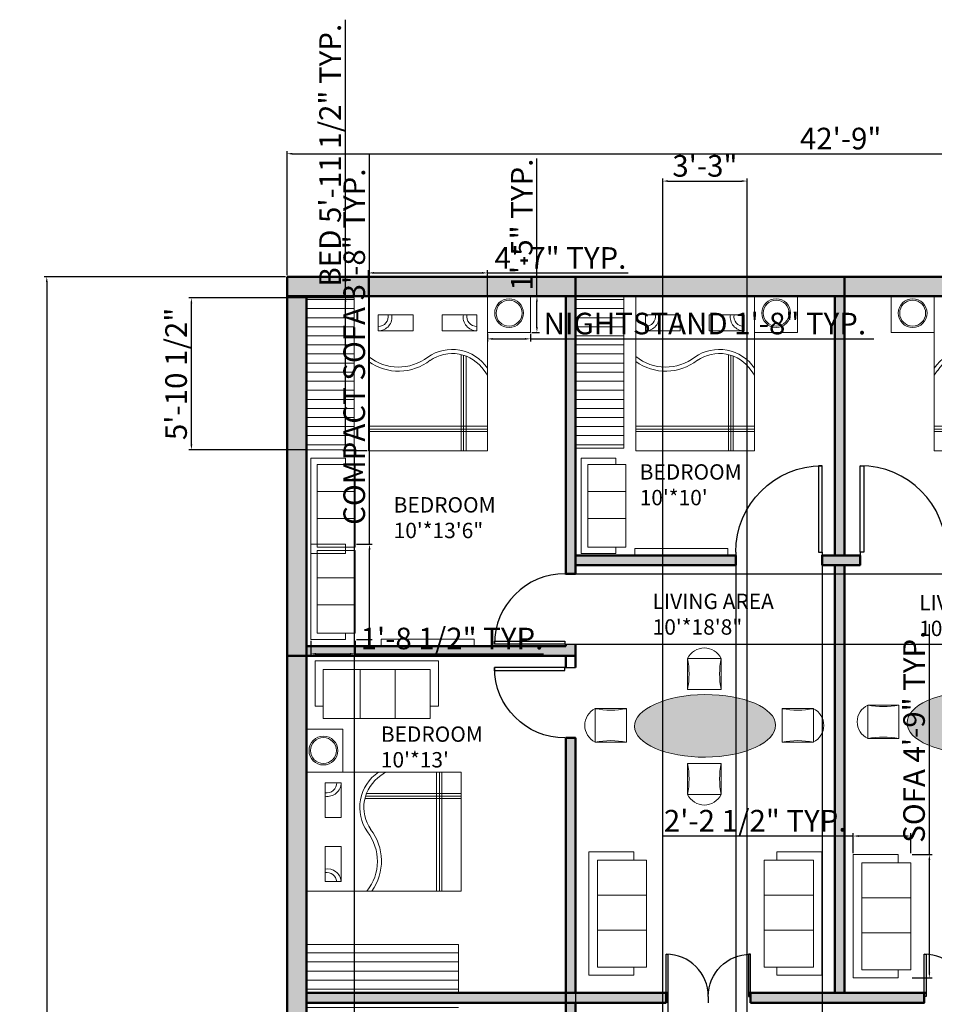
# Model space of a CAD drawing. Units: inches. Extents: x 1477 to 2233, y 1388 to 2326.
# Tile 3 of 4: x 1477 to 1901, y 1870 to 2326. Entities that reach past the tile are written whole.
import ezdxf

# ---------------------------------------------------------------- set-up
doc = ezdxf.new("R2010")
doc.units = ezdxf.units.IN
for name, color, linetype, lineweight in [('A-ANNO-DIMS', 2, 'Continuous', 18), ('A-AREA-IDEN', 7, 'Continuous', 18), ('A-DOOR', 4, 'Continuous', 25), ('A-EQPM', 8, 'Continuous', 18), ('A-FURN-PATT', 9, 'Continuous', 13), ('A-WALL-PATT', 10, 'Continuous', 13), ('bed', 200, 'Continuous', 18), ('book', 104, 'Continuous', 18), ('dining', 220, 'Continuous', 18), ('sofa', 130, 'Continuous', 18), ('table', 40, 'Continuous', 18), ('wall', 10, 'Continuous', 50)]:
    doc.layers.add(name, color=color, linetype=linetype, lineweight=lineweight)
doc.styles.get("Standard").update_dxf_attribs({"font": 'arial.ttf'})
doc.dimstyles.new('ISO-25', dxfattribs={"dimtxt": 10, "dimasz": 2.5, "dimexe": 1.25, "dimexo": 0.625, "dimtad": 1, "dimdec": 0, "dimlunit": 4, "dimtxsty": 'Standard', "dimcen": 2.5, "dimadec": 0, "dimazin": 0, "dimtfac": 1, "dimtdec": 0, "dimtmove": 0, "dimatfit": 3, "dimfxl": 1, "dimarcsym": 0})

# ---------------------------------------------------------------- blocks, each defined once
blk = doc.blocks.new('*U2')
for p, q in [((0, 0), (0, -6)), ((40, 0), (40, -6))]:
    blk.add_line(p, q)
blk.add_lwpolyline([(0, 0), (0, 40), (1.75, 40), (1.75, 0)], close=True)
blk.add_arc((0, 0), 40, 0, 90)
blk = doc.blocks.new('*D4')
at = {"layer": 'A-ANNO-DIMS', "color": 0, "lineweight": -2, "transparency": 16777216}
for p, q in [((1601.11, 2207.8), (1601.11, 2265.33)), ((2113.61, 2207.8), (2113.61, 2265.33)), ((1603.61, 2264.08), (2111.11, 2264.08))]:
    blk.add_line(p, q, dxfattribs=at)
at = {"layer": 'A-ANNO-DIMS', "color": 0, "transparency": 16777216}
for points in [[(1603.61, 2264.5), (1603.61, 2263.66), (1601.11, 2264.08)], [(2111.11, 2264.5), (2111.11, 2263.66), (2113.61, 2264.08)]]:
    blk.add_solid(points, dxfattribs=at)
at = {"layer": 'Defpoints', "color": 0, "transparency": 16777216}
for p in [(2113.61, 2264.08), (1601.11, 2207.17), (2113.61, 2207.17)]:
    blk.add_point(p, dxfattribs=at)
at = {"layer": 'A-ANNO-DIMS', "color": 0, "transparency": 16777216, "insert": (1857.36, 2269.81), "char_height": 10, "attachment_point": 5}
blk.add_mtext('42\'-9"', dxfattribs=at)
blk = doc.blocks.new('*D5')
at = {"layer": 'A-ANNO-DIMS', "color": 0, "lineweight": -2, "transparency": 16777216}
for p, q in [((1600.48, 2207.17), (1488.68, 2207.17)), ((1489.93, 2204.67), (1489.93, 1443.67)), ((1600.48, 1441.17), (1488.68, 1441.17))]:
    blk.add_line(p, q, dxfattribs=at)
at = {"layer": 'A-ANNO-DIMS', "color": 0, "transparency": 16777216}
for points in [[(1489.51, 2204.67), (1490.35, 2204.67), (1489.93, 2207.17)], [(1489.51, 1443.67), (1490.35, 1443.67), (1489.93, 1441.17)]]:
    blk.add_solid(points, dxfattribs=at)
at = {"layer": 'Defpoints', "color": 0, "transparency": 16777216}
for p in [(1601.11, 2207.17), (1489.93, 1441.17), (1601.11, 1441.17)]:
    blk.add_point(p, dxfattribs=at)
at = {"layer": 'A-ANNO-DIMS', "color": 0, "transparency": 16777216, "insert": (1484.2, 1824.17), "char_height": 10, "attachment_point": 5, "rotation": 90}
blk.add_mtext('63\'-10"', dxfattribs=at)
blk = doc.blocks.new('BED-DOUBLE')
for p, q in [((42.9, 44.24), (42.9, 44.54)), ((42.9, 44.24), (42.9, 0)), ((43.98, 44.24), (43.98, 0)), ((45.09, 43.85), (45.09, 0)), ((53.44, 37.23), (54.99, 35.03)), ((0, 11.42), (54.99, 11.42)), ((0, 10.1), (54.99, 10.1)), ((0, 8.97), (54.99, 8.97))]:
    blk.add_line(p, q)
for points in [[(0, 71.61), (54.99, 71.61), (54.99, 0), (0, 0)], [(4.46, 63.01), (20.6, 63.01), (20.6, 55.57), (4.46, 55.57)], [(50.13, 63.01), (34, 63.01), (34, 55.57), (50.13, 55.57)]]:
    blk.add_lwpolyline(points, close=True)
for centre, radius, start, end in [((4.46, 61.93), 6.36, 270, 9.8305), ((4.46, 62.26), 4.68, 270, 9.2541), ((50.13, 61.93), 6.36, 170.1695, 270), ((50.13, 62.26), 4.68, 170.7459, 270), ((38.65, 27.17), 19.76, 34.2245, 124.798), ((13.85, 60.88), 22.1, 231.1871, 307.7214), ((13.85, 60.88), 23.99, 234.7235, 307.7214), ((38.65, 27.17), 17.88, 34.2245, 124.798)]:
    blk.add_arc(centre, radius, start, end)
blk = doc.blocks.new('BED-DOUBLE-ALT')
for p, q in [((8.97, 0), (8.97, 54.99)), ((10.1, 0), (10.1, 54.99)), ((11.42, 0), (11.42, 54.99)), ((37.23, 53.44), (35.03, 54.99)), ((43.85, 45.09), (0, 45.09)), ((44.24, 43.98), (0, 43.98)), ((44.24, 42.9), (0, 42.9)), ((44.24, 42.9), (44.54, 42.9))]:
    blk.add_line(p, q)
for points in [[(71.61, 0), (71.61, 54.99), (0, 54.99), (0, 0)], [(63.01, 50.13), (63.01, 34), (55.57, 34), (55.57, 50.13)], [(63.01, 4.46), (63.01, 20.6), (55.57, 20.6), (55.57, 4.46)]]:
    blk.add_lwpolyline(points, close=True)
for centre, radius, start, end in [((27.17, 38.65), 19.76, 325.202, 55.7755), ((27.17, 38.65), 17.88, 325.202, 55.7755), ((61.93, 50.13), 6.36, 180, 279.8305), ((62.26, 50.13), 4.68, 180, 279.2541), ((60.88, 13.85), 23.99, 142.2786, 215.2765), ((60.88, 13.85), 22.1, 142.2786, 218.8129), ((61.93, 3.93), 6.36, 80.1695, 175.1865), ((62.26, 3.93), 4.68, 80.7459, 173.4549)]:
    blk.add_arc(centre, radius, start, end)
blk = doc.blocks.new('NIGHTSTAND-LAMP')
blk.add_lwpolyline([(0, 16.8), (19.92, 16.8), (19.92, 0), (0, 0)], close=True)
for radius in [6.66, 6]:
    blk.add_circle((10.02, 8.94), radius)
blk = doc.blocks.new('SOFA-COMPACT')
for p, q in [((0, 0), (0, 44.13)), ((16.12, 44.13), (0, 44.13)), ((16.12, 41.13), (16.12, 44.13)), ((3.06, 28.6), (20.62, 28.6)), ((3.06, 16.11), (20.62, 16.11)), ((16.12, 2.91), (16.12, 0)), ((16.12, 0), (0, 0))]:
    blk.add_line(p, q)
blk.add_lwpolyline([(20.62, 2.91), (3.06, 2.91), (3.06, 41.13), (20.62, 41.13)], close=True)
blk = doc.blocks.new('SOFA-COMPACT-ALT')
for p, q in [((0, 4.5), (0, 20.62)), ((0, 20.62), (44.13, 20.62)), ((44.13, 4.5), (44.13, 20.62)), ((16.11, 17.56), (16.11, 0)), ((28.61, 17.56), (28.61, 0)), ((2.91, 4.5), (0, 4.5)), ((1.29, 4.5), (2.91, 4.5)), ((41.13, 4.5), (44.13, 4.5))]:
    blk.add_line(p, q)
blk.add_lwpolyline([(2.91, 0), (2.91, 17.56), (41.13, 17.56), (41.13, 0)], close=True)
blk = doc.blocks.new('SOFA-STANDARD-ALT')
for p, q in [((0, 26.7), (57.14, 26.7)), ((0, 26.7), (0, 5.83)), ((57.14, 5.83), (57.14, 26.7)), ((20.86, 22.74), (20.86, 0)), ((37.04, 22.74), (37.04, 0)), ((3.76, 5.83), (0, 5.83)), ((53.26, 5.83), (57.14, 5.83))]:
    blk.add_line(p, q)
blk.add_lwpolyline([(3.76, 0), (3.76, 22.74), (53.26, 22.74), (53.26, 0)], close=True)
blk = doc.blocks.new('CHAIR-DINING')
blk.add_lwpolyline([(0, 0), (15.48, 0), (15.48, 14.4), (0, 14.4)], close=True)
for centre, radius, start, end in [((7.74, 10.64), 8.6, 25.8733, 154.1267), ((-38.59, 7.2), 39.26, 349.434, 10.566), ((53.9, 7.2), 39.09, 169.3873, 190.6127)]:
    blk.add_arc(centre, radius, start, end)
blk = doc.blocks.new('*D17')
at = {"layer": 'A-ANNO-DIMS', "color": 0, "lineweight": -2, "transparency": 16777216}
for p, q in [((1693.87, 2180.75), (1693.87, 2177.14)), ((1696.37, 2178.39), (1711.29, 2178.39)), ((1713.79, 2180.75), (1713.79, 2177.14)), ((1713.79, 2178.39), (1872.69, 2178.39))]:
    blk.add_line(p, q, dxfattribs=at)
at = {"layer": 'A-ANNO-DIMS', "color": 0, "transparency": 16777216}
for points in [[(1696.37, 2178.8), (1696.37, 2177.97), (1693.87, 2178.39)], [(1711.29, 2178.8), (1711.29, 2177.97), (1713.79, 2178.39)]]:
    blk.add_solid(points, dxfattribs=at)
at = {"layer": 'Defpoints', "color": 0, "transparency": 16777216}
for p in [(1693.87, 2181.38), (1713.79, 2181.38), (1713.79, 2178.39)]:
    blk.add_point(p, dxfattribs=at)
at = {"layer": 'A-ANNO-DIMS', "color": 0, "transparency": 16777216, "insert": (1794.49, 2184.18), "char_height": 10, "attachment_point": 5}
blk.add_mtext('NIGHTSTAND 1\'-8" TYP.', dxfattribs=at)
blk = doc.blocks.new('*D18')
at = {"layer": 'A-ANNO-DIMS', "color": 0, "lineweight": -2, "transparency": 16777216}
for p, q in [((1716.78, 2198.17), (1716.78, 2261.94)), ((1714.41, 2198.17), (1718.03, 2198.17)), ((1716.78, 2183.88), (1716.78, 2195.67)), ((1714.41, 2181.38), (1718.03, 2181.38))]:
    blk.add_line(p, q, dxfattribs=at)
at = {"layer": 'A-ANNO-DIMS', "color": 0, "transparency": 16777216}
for points in [[(1716.36, 2195.67), (1717.19, 2195.67), (1716.78, 2198.17)], [(1716.36, 2183.88), (1717.19, 2183.88), (1716.78, 2181.38)]]:
    blk.add_solid(points, dxfattribs=at)
at = {"layer": 'Defpoints', "color": 0, "transparency": 16777216}
for p in [(1713.79, 2198.17), (1716.78, 2198.17), (1713.79, 2181.38)]:
    blk.add_point(p, dxfattribs=at)
at = {"layer": 'A-ANNO-DIMS', "color": 0, "transparency": 16777216, "insert": (1711.05, 2231.3), "char_height": 10, "attachment_point": 5, "rotation": 90}
blk.add_mtext('1\'-5" TYP.', dxfattribs=at)
blk = doc.blocks.new('*D19')
at = {"layer": 'A-ANNO-DIMS', "color": 0, "lineweight": -2, "transparency": 16777216}
for p, q in [((1898.42, 1939.74), (1898.42, 2046.31)), ((1890.47, 1939.74), (1899.67, 1939.74)), ((1898.42, 1885.1), (1898.42, 1937.24)), ((1890.47, 1882.6), (1899.67, 1882.6))]:
    blk.add_line(p, q, dxfattribs=at)
at = {"layer": 'A-ANNO-DIMS', "color": 0, "transparency": 16777216}
for points in [[(1898, 1937.24), (1898.83, 1937.24), (1898.42, 1939.74)], [(1898, 1885.1), (1898.83, 1885.1), (1898.42, 1882.6)]]:
    blk.add_solid(points, dxfattribs=at)
at = {"layer": 'Defpoints', "color": 0, "transparency": 16777216}
for p in [(1889.85, 1939.74), (1898.42, 1939.74), (1889.85, 1882.6)]:
    blk.add_point(p, dxfattribs=at)
at = {"layer": 'A-ANNO-DIMS', "color": 0, "transparency": 16777216, "insert": (1892.62, 1994.27), "char_height": 10, "attachment_point": 5, "rotation": 90}
blk.add_mtext('SOFA 4\'-9" TYP.', dxfattribs=at)
blk = doc.blocks.new('*D20')
at = {"layer": 'A-ANNO-DIMS', "color": 0, "lineweight": -2, "transparency": 16777216}
for p, q in [((1863.14, 1948.31), (1774.97, 1948.31)), ((1863.14, 1940.36), (1863.14, 1949.56)), ((1887.35, 1948.31), (1865.64, 1948.31)), ((1889.85, 1940.36), (1889.85, 1949.56))]:
    blk.add_line(p, q, dxfattribs=at)
at = {"layer": 'A-ANNO-DIMS', "color": 0, "transparency": 16777216}
for points in [[(1865.64, 1948.72), (1865.64, 1947.89), (1863.14, 1948.31)], [(1887.35, 1948.72), (1887.35, 1947.89), (1889.85, 1948.31)]]:
    blk.add_solid(points, dxfattribs=at)
at = {"layer": 'Defpoints', "color": 0, "transparency": 16777216}
for p in [(1863.14, 1948.31), (1863.14, 1939.74), (1889.85, 1939.74)]:
    blk.add_point(p, dxfattribs=at)
at = {"layer": 'A-ANNO-DIMS', "color": 0, "transparency": 16777216, "insert": (1817.81, 1954.1), "char_height": 10, "attachment_point": 5}
blk.add_mtext('2\'-2 1/2" TYP.', dxfattribs=at)
blk = doc.blocks.new('*D23')
at = {"layer": 'A-ANNO-DIMS', "color": 0, "lineweight": -2, "transparency": 16777216}
for p, q in [((1628.13, 2198.17), (1628.13, 2326.11)), ((1638.25, 2198.17), (1626.88, 2198.17)), ((1628.13, 2129.06), (1628.13, 2195.67)), ((1638.25, 2126.56), (1626.88, 2126.56))]:
    blk.add_line(p, q, dxfattribs=at)
at = {"layer": 'A-ANNO-DIMS', "color": 0, "transparency": 16777216}
for points in [[(1627.72, 2195.67), (1628.55, 2195.67), (1628.13, 2198.17)], [(1627.72, 2129.06), (1628.55, 2129.06), (1628.13, 2126.56)]]:
    blk.add_solid(points, dxfattribs=at)
at = {"layer": 'Defpoints', "color": 0, "transparency": 16777216}
for p in [(1628.13, 2198.17), (1638.87, 2198.17), (1638.87, 2126.56)]:
    blk.add_point(p, dxfattribs=at)
at = {"layer": 'A-ANNO-DIMS', "color": 0, "transparency": 16777216, "insert": (1622.34, 2263.39), "char_height": 10, "attachment_point": 5, "rotation": 90}
blk.add_mtext('BED 5\'-11 1/2" TYP.', dxfattribs=at)
blk = doc.blocks.new('*D24')
at = {"layer": 'A-ANNO-DIMS', "color": 0, "lineweight": -2, "transparency": 16777216}
for p, q in [((1638.87, 2198.8), (1638.87, 2210.16)), ((1693.87, 2198.8), (1693.87, 2210.16)), ((1641.37, 2208.91), (1691.37, 2208.91)), ((1693.87, 2208.91), (1758.98, 2208.91))]:
    blk.add_line(p, q, dxfattribs=at)
at = {"layer": 'A-ANNO-DIMS', "color": 0, "transparency": 16777216}
for points in [[(1641.37, 2209.33), (1641.37, 2208.5), (1638.87, 2208.91)], [(1691.37, 2209.33), (1691.37, 2208.5), (1693.87, 2208.91)]]:
    blk.add_solid(points, dxfattribs=at)
at = {"layer": 'Defpoints', "color": 0, "transparency": 16777216}
for p in [(1693.87, 2208.91), (1638.87, 2198.17), (1693.87, 2198.17)]:
    blk.add_point(p, dxfattribs=at)
at = {"layer": 'A-ANNO-DIMS', "color": 0, "transparency": 16777216, "insert": (1727.67, 2214.54), "char_height": 10, "attachment_point": 5}
blk.add_mtext('4\'-7" TYP.', dxfattribs=at)
blk = doc.blocks.new('*D31')
at = {"layer": 'A-ANNO-DIMS', "color": 0, "lineweight": -2, "transparency": 16777216}
for p, q in [((1639.31, 2083.39), (1639.31, 2263.63)), ((1633.32, 2083.39), (1640.56, 2083.39)), ((1639.31, 2041.76), (1639.31, 2080.89)), ((1633.32, 2039.26), (1640.56, 2039.26))]:
    blk.add_line(p, q, dxfattribs=at)
at = {"layer": 'A-ANNO-DIMS', "color": 0, "transparency": 16777216}
for points in [[(1638.9, 2080.89), (1639.73, 2080.89), (1639.31, 2083.39)], [(1638.9, 2041.76), (1639.73, 2041.76), (1639.31, 2039.26)]]:
    blk.add_solid(points, dxfattribs=at)
at = {"layer": 'Defpoints', "color": 0, "transparency": 16777216}
for p in [(1632.69, 2083.39), (1639.31, 2083.39), (1632.69, 2039.26)]:
    blk.add_point(p, dxfattribs=at)
at = {"layer": 'A-ANNO-DIMS', "color": 0, "transparency": 16777216, "insert": (1633.51, 2174.76), "char_height": 10, "attachment_point": 5, "rotation": 90}
blk.add_mtext('COMPACT SOFA 3\'-8" TYP.', dxfattribs=at)
blk = doc.blocks.new('*D32')
at = {"layer": 'A-ANNO-DIMS', "color": 0, "lineweight": -2, "transparency": 16777216}
for p, q in [((1612.07, 2038.63), (1612.07, 2031.39)), ((1632.69, 2038.63), (1632.69, 2031.39)), ((1614.57, 2032.64), (1630.19, 2032.64)), ((1632.69, 2032.64), (1719.76, 2032.64))]:
    blk.add_line(p, q, dxfattribs=at)
at = {"layer": 'A-ANNO-DIMS', "color": 0, "transparency": 16777216}
for points in [[(1614.57, 2033.05), (1614.57, 2032.22), (1612.07, 2032.64)], [(1630.19, 2033.05), (1630.19, 2032.22), (1632.69, 2032.64)]]:
    blk.add_solid(points, dxfattribs=at)
at = {"layer": 'Defpoints', "color": 0, "transparency": 16777216}
for p in [(1612.07, 2039.26), (1632.69, 2039.26), (1632.69, 2032.64)]:
    blk.add_point(p, dxfattribs=at)
at = {"layer": 'A-ANNO-DIMS', "color": 0, "transparency": 16777216, "insert": (1677.47, 2038.43), "char_height": 10, "attachment_point": 5}
blk.add_mtext('1\'-8 1/2" TYP.', dxfattribs=at)
blk = doc.blocks.new('*D40')
at = {"layer": 'A-ANNO-DIMS', "color": 0, "lineweight": -2, "transparency": 16777216}
for p, q in [((2157.86, 2069.66), (2157.86, 2123.47)), ((1730.73, 2069.66), (2159.11, 2069.66)), ((2157.86, 2039.56), (2157.86, 2067.16)), ((1730.73, 2037.06), (2159.11, 2037.06))]:
    blk.add_line(p, q, dxfattribs=at)
at = {"layer": 'A-ANNO-DIMS', "color": 0, "transparency": 16777216}
for points in [[(2157.44, 2067.16), (2158.27, 2067.16), (2157.86, 2069.66)], [(2157.44, 2039.56), (2158.27, 2039.56), (2157.86, 2037.06)]]:
    blk.add_solid(points, dxfattribs=at)
at = {"layer": 'Defpoints', "color": 0, "transparency": 16777216}
for p in [(1730.11, 2069.66), (2157.86, 2069.66), (1730.11, 2037.06)]:
    blk.add_point(p, dxfattribs=at)
at = {"layer": 'A-ANNO-DIMS', "color": 0, "transparency": 16777216, "insert": (2152.06, 2097.82), "char_height": 10, "attachment_point": 5, "rotation": 90}
blk.add_mtext('2\'-8 1/2"', dxfattribs=at)
blk = doc.blocks.new('*D41')
at = {"layer": 'A-ANNO-DIMS', "color": 0, "lineweight": -2, "transparency": 16777216}
for p, q in [((1610.11, 2126.39), (1610.11, 1395.67)), ((1632.2, 2126.39), (1632.2, 1395.67)), ((1612.61, 1396.92), (1629.7, 1396.92)), ((1632.2, 1396.92), (1669.36, 1396.92))]:
    blk.add_line(p, q, dxfattribs=at)
at = {"layer": 'A-ANNO-DIMS', "color": 0, "transparency": 16777216}
for points in [[(1612.61, 1397.34), (1612.61, 1396.51), (1610.11, 1396.92)], [(1629.7, 1397.34), (1629.7, 1396.51), (1632.2, 1396.92)]]:
    blk.add_solid(points, dxfattribs=at)
at = {"layer": 'Defpoints', "color": 0, "transparency": 16777216}
for p in [(1610.11, 2127.01), (1632.2, 2127.01), (1632.2, 1396.92)]:
    blk.add_point(p, dxfattribs=at)
at = {"layer": 'A-ANNO-DIMS', "color": 0, "transparency": 16777216, "insert": (1652.03, 1402.65), "char_height": 10, "attachment_point": 5}
blk.add_mtext('1\'-10"', dxfattribs=at)
blk = doc.blocks.new('*D42')
at = {"layer": 'A-ANNO-DIMS', "color": 0, "lineweight": -2, "transparency": 16777216}
for p, q in [((1609.48, 2197.32), (1555.61, 2197.32)), ((1556.86, 2129.51), (1556.86, 2194.82)), ((1609.48, 2127.01), (1555.61, 2127.01))]:
    blk.add_line(p, q, dxfattribs=at)
at = {"layer": 'A-ANNO-DIMS', "color": 0, "transparency": 16777216}
for points in [[(1556.44, 2194.82), (1557.27, 2194.82), (1556.86, 2197.32)], [(1556.44, 2129.51), (1557.27, 2129.51), (1556.86, 2127.01)]]:
    blk.add_solid(points, dxfattribs=at)
at = {"layer": 'Defpoints', "color": 0, "transparency": 16777216}
for p in [(1556.86, 2197.32), (1610.11, 2197.32), (1610.11, 2127.01)]:
    blk.add_point(p, dxfattribs=at)
at = {"layer": 'A-ANNO-DIMS', "color": 0, "transparency": 16777216, "insert": (1551.06, 2162.17), "char_height": 10, "attachment_point": 5, "rotation": 90}
blk.add_mtext('5\'-10 1/2"', dxfattribs=at)
blk = doc.blocks.new('*D45')
at = {"layer": 'A-ANNO-DIMS', "color": 0, "lineweight": -2, "transparency": 16777216}
for p, q in [((1601.11, 2031.05), (1601.11, 1395.67)), ((1610.11, 2031.05), (1610.11, 1395.67)), ((1603.61, 1396.92), (1607.61, 1396.92)), ((1610.11, 1396.92), (1640.44, 1396.92))]:
    blk.add_line(p, q, dxfattribs=at)
at = {"layer": 'A-ANNO-DIMS', "color": 0, "transparency": 16777216}
for points in [[(1603.61, 1397.34), (1603.61, 1396.51), (1601.11, 1396.92)], [(1607.61, 1397.34), (1607.61, 1396.51), (1610.11, 1396.92)]]:
    blk.add_solid(points, dxfattribs=at)
at = {"layer": 'Defpoints', "color": 0, "transparency": 16777216}
for p in [(1601.11, 2031.67), (1610.11, 2031.67), (1610.11, 1396.92)]:
    blk.add_point(p, dxfattribs=at)
at = {"layer": 'A-ANNO-DIMS', "color": 0, "transparency": 16777216, "insert": (1626.52, 1402.65), "char_height": 10, "attachment_point": 5}
blk.add_mtext('0\'-9"', dxfattribs=at)
blk = doc.blocks.new('*D47')
at = {"layer": 'A-ANNO-DIMS', "color": 0, "lineweight": -2, "transparency": 16777216}
for p, q in [((1775, 1723.3), (1775, 2252.67)), ((1777.5, 2251.42), (1811.54, 2251.42)), ((1814.04, 1723.3), (1814.04, 2252.67))]:
    blk.add_line(p, q, dxfattribs=at)
at = {"layer": 'A-ANNO-DIMS', "color": 0, "transparency": 16777216}
for points in [[(1777.5, 2251.84), (1777.5, 2251.01), (1775, 2251.42)], [(1811.54, 2251.84), (1811.54, 2251.01), (1814.04, 2251.42)]]:
    blk.add_solid(points, dxfattribs=at)
at = {"layer": 'Defpoints', "color": 0, "transparency": 16777216}
for p in [(1814.04, 2251.42), (1775, 1722.67), (1814.04, 1722.67)]:
    blk.add_point(p, dxfattribs=at)
at = {"layer": 'A-ANNO-DIMS', "color": 0, "transparency": 16777216, "insert": (1794.52, 2257.16), "char_height": 10, "attachment_point": 5}
blk.add_mtext('3\'-3"', dxfattribs=at)
blk = doc.blocks.new('*D48')
at = {"layer": 'A-ANNO-DIMS', "color": 0, "lineweight": -2, "transparency": 16777216}
for p, q in [((1734.61, 1875.05), (1734.61, 1395.67)), ((1777.43, 1875.05), (1777.43, 1395.67)), ((1737.11, 1396.92), (1774.93, 1396.92))]:
    blk.add_line(p, q, dxfattribs=at)
at = {"layer": 'A-ANNO-DIMS', "color": 0, "transparency": 16777216}
for points in [[(1737.11, 1397.34), (1737.11, 1396.51), (1734.61, 1396.92)], [(1774.93, 1397.34), (1774.93, 1396.51), (1777.43, 1396.92)]]:
    blk.add_solid(points, dxfattribs=at)
at = {"layer": 'Defpoints', "color": 0, "transparency": 16777216}
for p in [(1734.61, 1875.67), (1777.43, 1875.67), (1777.43, 1396.92)]:
    blk.add_point(p, dxfattribs=at)
at = {"layer": 'A-ANNO-DIMS', "color": 0, "transparency": 16777216, "insert": (1756.02, 1402.66), "char_height": 10, "attachment_point": 5}
blk.add_mtext('3\'-7"', dxfattribs=at)
blk = doc.blocks.new('*D49')
at = {"layer": 'A-ANNO-DIMS', "color": 0, "lineweight": -2, "transparency": 16777216}
for p, q in [((1808.79, 2077.55), (1808.79, 1395.67)), ((1848.79, 2077.55), (1848.79, 1395.67)), ((1811.29, 1396.92), (1846.29, 1396.92))]:
    blk.add_line(p, q, dxfattribs=at)
at = {"layer": 'A-ANNO-DIMS', "color": 0, "transparency": 16777216}
for points in [[(1811.29, 1397.34), (1811.29, 1396.51), (1808.79, 1396.92)], [(1846.29, 1397.34), (1846.29, 1396.51), (1848.79, 1396.92)]]:
    blk.add_solid(points, dxfattribs=at)
at = {"layer": 'Defpoints', "color": 0, "transparency": 16777216}
for p in [(1808.79, 2078.17), (1848.79, 2078.17), (1848.79, 1396.92)]:
    blk.add_point(p, dxfattribs=at)
at = {"layer": 'A-ANNO-DIMS', "color": 0, "transparency": 16777216, "insert": (1828.79, 1402.66), "char_height": 10, "attachment_point": 5}
blk.add_mtext('3\'-4"', dxfattribs=at)

msp = doc.modelspace()

# ---------------------------------------------------------------- hatches: boundary and pattern name
at = {"layer": 'A-FURN-PATT'}
h = msp.add_hatch(dxfattribs=at)
h.set_pattern_fill('_USER', color=256, scale=4.2, pattern_type=0)
h.set_pattern_definition([(0, (0, 0), (0, 4.2), [])])
h.paths.add_polyline_path([(1632.2, 2197.32), (1610.11, 2197.32), (1610.11, 2127.01), (1632.2, 2127.01)])
h.paths.add_polyline_path([(1757.03, 2198.17), (1734.93, 2198.17), (1734.93, 2127.87), (1757.03, 2127.87)])
h.paths.add_polyline_path([(1979.11, 2198.17), (1957.06, 2198.17), (1957.06, 2127.87), (1979.11, 2127.87)])
h.paths.add_polyline_path([(2104.61, 2198.17), (2082.56, 2198.17), (2082.56, 2127.87), (2104.61, 2127.87)])
h.paths.add_polyline_path([(2104.61, 1897.77), (2034.3, 1897.77), (2034.3, 1875.67), (2104.61, 1875.67)])
h.paths.add_polyline_path([(1680.41, 1898.15), (1610.11, 1898.15), (1610.11, 1876.06), (1680.41, 1876.06)])
h.paths.add_polyline_path([(1680.41, 1869.67), (1610.11, 1869.67), (1610.11, 1847.57), (1680.41, 1847.57)])
h.paths.add_polyline_path([(1632.2, 1521.19), (1610.11, 1521.19), (1610.11, 1450.88), (1632.2, 1450.88)])
h.paths.add_polyline_path([(1854.34, 1520.43), (1832.24, 1520.43), (1832.24, 1450.17), (1854.34, 1450.17)])
h = msp.add_hatch(color=256, dxfattribs=at)
h.dxf.hatch_style = 1
edge = h.paths.add_edge_path()
edge.add_ellipse((1794.61, 1999.29), major_axis=(32.65, 0.27), ratio=0.443592, start_angle=0, end_angle=360)
edge = h.paths.add_edge_path()
edge.add_ellipse((1920.72, 2000.93), major_axis=(32.65, 0.27), ratio=0.443592, start_angle=0, end_angle=360)
edge = h.paths.add_edge_path()
edge.add_ellipse((1854.61, 1811.96), major_axis=(32.65, 0.27), ratio=0.443592, start_angle=0, end_angle=360)
edge = h.paths.add_edge_path()
edge.add_ellipse((1749.3, 1659.55), major_axis=(32.65, 0.27), ratio=0.443592, start_angle=0, end_angle=360)
at = {"layer": 'A-WALL-PATT'}
h = msp.add_hatch(color=256, dxfattribs=at)
h.dxf.hatch_style = 1
h.paths.add_polyline_path([(2104.61, 2036.17), (1979.11, 2036.17), (1979.11, 2031.67), (2104.61, 2031.67)])
h.paths.add_polyline_path([(1983.61, 2031.67), (1979.11, 2031.67), (1979.11, 2027.53), (1983.61, 2027.53)])
h.paths.add_polyline_path([(1983.61, 2037.7), (1979.11, 2037.7), (1979.11, 2036.17), (1983.61, 2036.17)])
h.paths.add_polyline_path([(2113.61, 2207.17), (2104.61, 2207.17), (2104.61, 2031.67), (2113.61, 2031.67)])
h.paths.add_polyline_path([(2104.61, 2207.17), (1859.11, 2207.17), (1859.11, 2198.17), (2104.61, 2198.17)])
h.paths.add_polyline_path([(1983.61, 2198.17), (1979.16, 2198.17), (1979.16, 2127.87), (1979.11, 2070.31), (1983.61, 2070.31)])
h.paths.add_polyline_path([(1979.11, 2078.17), (1906.33, 2078.17), (1906.33, 2073.67), (1979.11, 2073.67)])
h.paths.add_polyline_path([(1859.11, 2198.17), (1854.61, 2198.17), (1854.61, 2078.17), (1859.11, 2078.17)])
h.paths.add_polyline_path([(1866.33, 2078.17), (1848.79, 2078.17), (1848.79, 2073.67), (1866.33, 2073.67)])
h.paths.add_polyline_path([(1859.11, 2207.17), (1734.61, 2207.17), (1734.61, 2198.17), (1859.11, 2198.17)])
h.paths.add_polyline_path([(1734.61, 2207.17), (1601.11, 2207.17), (1601.11, 2198.17), (1610.11, 2198.17), (1734.61, 2198.17)])
h.paths.add_polyline_path([(1734.61, 2198.17), (1730.11, 2198.17), (1730.11, 2069.66), (1734.61, 2069.66)])
h.paths.add_polyline_path([(1808.79, 2078.17), (1734.61, 2078.17), (1734.61, 2073.67), (1808.79, 2073.67)])
h.paths.add_polyline_path([(1610.11, 2198.17), (1601.11, 2198.17), (1601.11, 1450.43), (1610.11, 1450.43)])
h.paths.add_polyline_path([(2104.61, 1450.43), (1854.61, 1450.43), (1854.61, 1450.17), (1854.34, 1450.13), (1832.24, 1450.13), (1830.34, 1450.13), (1830.34, 1450.03), (1775.35, 1450.03), (1755.43, 1450.03), (1713.79, 1450.14), (1713.79, 1450.03), (1693.87, 1450.03), (1638.87, 1450.03), (1610.11, 1450.17), (1610.11, 1450.43), (1601.11, 1450.43), (1601.11, 1441.17), (2104.61, 1441.17)])
h.paths.add_polyline_path([(2113.61, 1871.17), (2104.61, 1871.17), (2104.61, 1441.17), (2113.61, 1441.17)])
h.paths.add_polyline_path([(1734.61, 1598.17), (1730.11, 1598.17), (1730.11, 1450.43), (1734.61, 1450.43)])
h = msp.add_hatch(color=256, dxfattribs=at)
h.dxf.hatch_style = 1
h.paths.add_polyline_path([(1859.11, 2073.67), (1854.61, 2073.67), (1854.61, 1875.67), (1859.11, 1875.67)])
h = msp.add_hatch(color=256, dxfattribs=at)
h.dxf.hatch_style = 1
h.paths.add_polyline_path([(1734.61, 2037.06), (1730.11, 2037.06), (1730.11, 2036.17), (1610.11, 2036.17), (1610.11, 2031.67), (1734.61, 2031.67)])
h.paths.add_polyline_path([(1983.61, 1994.92), (1979.11, 1994.92), (1979.11, 1875.67), (1983.61, 1875.67)])
h = msp.add_hatch(color=256, dxfattribs=at)
h.dxf.hatch_style = 1
h.paths.add_polyline_path([(1734.61, 1993.71), (1730.11, 1993.71), (1730.11, 1875.67), (1734.61, 1875.67)])
h.paths.add_polyline_path([(1730.11, 1875.67), (1610.11, 1875.67), (1610.11, 1871.17), (1730.11, 1871.17)])
h.paths.add_polyline_path([(1776.57, 1875.67), (1730.11, 1875.67), (1730.11, 1871.17), (1776.57, 1871.17)])
h.paths.add_polyline_path([(1896.07, 1875.67), (1815.6, 1875.67), (1815.6, 1871.17), (1896.07, 1871.17)])
h.paths.add_polyline_path([(2104.61, 1875.67), (1935.11, 1875.67), (1935.11, 1871.17), (2104.61, 1871.17)])
h.paths.add_polyline_path([(1734.61, 1871.17), (1730.11, 1871.17), (1730.11, 1727.17), (1734.61, 1727.17)])
h.paths.add_polyline_path([(1775, 1727.17), (1726.93, 1727.17), (1726.93, 1722.67), (1775, 1722.67)])
h.paths.add_polyline_path([(1880.17, 1727.17), (1814.04, 1727.17), (1814.04, 1722.67), (1880.17, 1722.67)])
h.paths.add_polyline_path([(1858.61, 1722.67), (1854.11, 1722.67), (1854.12, 1598.17), (1858.61, 1598.17)])
h.paths.add_polyline_path([(1854.12, 1602.67), (1780.08, 1602.67), (1780.08, 1598.17), (1854.12, 1598.17)])
h.paths.add_polyline_path([(1740.08, 1602.67), (1722.89, 1602.67), (1722.89, 1598.17), (1740.08, 1598.17)])
h.paths.add_polyline_path([(1682.89, 1602.67), (1610.11, 1602.67), (1610.11, 1598.17), (1682.89, 1598.17)])
h.paths.add_polyline_path([(1859.11, 1598.17), (1854.61, 1598.17), (1854.61, 1450.43), (1859.11, 1450.43)])
h.paths.add_polyline_path([(2104.61, 1727.17), (1960.17, 1727.17), (1960.17, 1722.67), (2104.61, 1722.67)])
h.paths.add_polyline_path([(2104.61, 1625.03), (1978.61, 1625.03), (1978.61, 1620.53), (2104.61, 1620.53)])

# ---------------------------------------------------------------- linework, layer by layer
at = {"layer": 'A-EQPM'}
for points in [[(1762.04, 2078.17), (1805.1, 2078.17), (1805.1, 2081.42), (1762.04, 2081.42)], [(1644.73, 2036.17), (1687.78, 2036.17), (1687.78, 2039.42), (1644.73, 2039.42)]]:
    msp.add_lwpolyline(points, close=True, dxfattribs=at)
at = {"layer": 'book'}
for points in [[(1632.2, 2197.32), (1610.11, 2197.32), (1610.11, 2127.01), (1632.2, 2127.01)], [(1757.03, 2198.17), (1734.93, 2198.17), (1734.93, 2127.87), (1757.03, 2127.87)], [(1610.11, 1898.15), (1610.11, 1876.06), (1680.41, 1876.06), (1680.41, 1898.15)]]:
    msp.add_lwpolyline(points, close=True, dxfattribs=at)
at = {"layer": 'dining'}
for centre in [(1920.72, 2000.93), (1794.61, 1999.29)]:
    msp.add_ellipse(centre, major_axis=(32.65, 0.27), ratio=0.443592, dxfattribs=at)
at = {"layer": 'wall'}
for p, q in [((1601.11, 2031.67), (1601.11, 2207.17)), ((1601.11, 2207.17), (1734.61, 2207.17)), ((1734.61, 2207.17), (1734.61, 2069.66)), ((1734.61, 2207.17), (1859.11, 2207.17)), ((1859.11, 2207.17), (1859.11, 2078.17)), ((1859.11, 2207.17), (1983.61, 2207.17)), ((1610.11, 2198.17), (1730.11, 2198.17)), ((1610.11, 2036.17), (1610.11, 2198.17)), ((1730.11, 2198.17), (1730.11, 2069.66)), ((1734.61, 2198.17), (1854.61, 2198.17)), ((1854.61, 2198.17), (1854.61, 2078.17)), ((1859.11, 2198.17), (1979.11, 2198.17)), ((1808.79, 2078.17), (1734.61, 2078.17)), ((1854.61, 2078.17), (1848.79, 2078.17)), ((1866.33, 2078.17), (1859.11, 2078.17)), ((1808.79, 2073.67), (1734.61, 2073.67)), ((1859.11, 2073.67), (1848.79, 2073.67)), ((1854.61, 2073.67), (1854.61, 1875.67)), ((1859.11, 2073.67), (1859.11, 1875.67)), ((1866.33, 2073.67), (1859.11, 2073.67)), ((1730.11, 2037.06), (1730.11, 2036.17)), ((1734.61, 2037.06), (1734.61, 2031.67)), ((1730.11, 2036.17), (1610.11, 2036.17)), ((1734.61, 2031.67), (1601.11, 2031.67)), ((1601.11, 2031.67), (1601.11, 1871.17)), ((1610.11, 2031.67), (1610.11, 1875.67)), ((1730.11, 2026.32), (1730.11, 2031.67)), ((1734.61, 2026.32), (1734.61, 2031.67)), ((1730.11, 1875.67), (1730.11, 1993.71)), ((1734.61, 1875.67), (1734.61, 1993.71)), ((1610.11, 1875.67), (1730.11, 1875.67)), ((1734.61, 1875.67), (1777.43, 1875.67)), ((1796.02, 1875.67), (1796.15, 1875.67)), ((1814.75, 1875.67), (1854.61, 1875.67)), ((1859.11, 1875.67), (1896.93, 1875.67)), ((1601.11, 1871.17), (1601.11, 1722.67)), ((1610.11, 1871.17), (1730.11, 1871.17)), ((1610.11, 1871.17), (1610.11, 1727.17)), ((1730.11, 1727.17), (1730.11, 1871.17)), ((1734.61, 1727.17), (1734.61, 1871.17)), ((1734.61, 1871.17), (1776.57, 1871.17)), ((1815.6, 1871.17), (1896.07, 1871.17))]:
    msp.add_line(p, q, dxfattribs=at)
for points in [[(1601.11, 2207.17), (2104.61, 2207.17), (2104.61, 2198.17), (1601.11, 2198.17)], [(1601.11, 1450.43), (1610.11, 1450.43), (1610.11, 2198.17), (1601.11, 2198.17)], [(1734.61, 2198.17), (1730.11, 2198.17), (1730.11, 2069.66), (1734.61, 2069.66)], [(1854.61, 2198.17), (1859.11, 2198.17), (1859.11, 2078.17), (1854.61, 2078.17)], [(1734.61, 2078.17), (1808.79, 2078.17), (1808.79, 2073.67), (1734.61, 2073.67)], [(1848.79, 2073.67), (1866.33, 2073.67), (1866.33, 2078.17), (1848.79, 2078.17)], [(1730.11, 1993.71), (1734.61, 1993.71), (1734.61, 1875.67), (1730.11, 1875.67)], [(1610.11, 1871.17), (1730.11, 1871.17), (1730.11, 1875.67), (1610.11, 1875.67)], [(1776.57, 1871.17), (1730.11, 1871.17), (1730.11, 1875.67), (1776.57, 1875.67)], [(1815.6, 1871.17), (1896.07, 1871.17), (1896.07, 1875.67), (1815.6, 1875.67)], [(1730.11, 1871.17), (1734.61, 1871.17), (1734.61, 1727.17), (1730.11, 1727.17)]]:
    msp.add_lwpolyline(points, close=True, dxfattribs=at)

# ---------------------------------------------------------------- block references
at = {"layer": 'A-DOOR', "xscale": -1}
msp.add_blockref('*U2', (1848.79, 2079.67), dxfattribs=at)
at = {"layer": 'A-DOOR'}
msp.add_blockref('*U2', (1866.33, 2079.67), dxfattribs=at)
at = {"layer": 'A-DOOR', "yscale": 0.8152383750006338, "zscale": 0.8152383750006338, "rotation": 90}
for p, xscale in [((1729.72, 2037.06), 0.8152383750006338), ((1729.72, 2026.32), -0.8152383750006338)]:
    msp.add_blockref('*U2', p, dxfattribs=dict(at, xscale=xscale))
at = {"layer": 'A-DOOR', "yscale": 0.4878891377503276, "zscale": 0.4878891377503276}
for p, xscale in [((1776.57, 1874.1), 0.4878891377503276), ((1815.6, 1874.1), -0.4878891377503276), ((1896.07, 1874.1), 0.4878891377503276)]:
    msp.add_blockref('*U2', p, dxfattribs=dict(at, xscale=xscale))
at = {"layer": 'bed'}
for p in [(1638.87, 2126.56), (1762.51, 2126.56)]:
    msp.add_blockref('BED-DOUBLE', p, dxfattribs=at)
at = {"layer": 'bed', "extrusion": (0, 0, -1), "zscale": -1}
for name, p in [('BED-DOUBLE', (-1955.7, 2126.56)), ('BED-DOUBLE-ALT', (-1681.72, 1922.84))]:
    msp.add_blockref(name, p, dxfattribs=at)
at = {"layer": 'dining'}
msp.add_blockref('CHAIR-DINING', (1786.51, 2016.11), dxfattribs=at)
at = {"layer": 'dining', "extrusion": (0, 0, -1), "zscale": -1}
for p, rotation in [((-1758.17, 2007.25), 269.9999999999997), ((-1884.28, 2008.9), 270.0000000000006), ((-1786.51, 1981.9), 180)]:
    msp.add_blockref('CHAIR-DINING', p, dxfattribs=dict(at, rotation=rotation))
at = {"layer": 'dining', "rotation": 270.0000000000008}
msp.add_blockref('CHAIR-DINING', (1830.32, 2007.25), dxfattribs=at)
at = {"layer": 'sofa'}
for name, p in [('SOFA-COMPACT', (1612.07, 2079.1)), ('SOFA-COMPACT', (1612.07, 2039.26)), ('SOFA-STANDARD-ALT', (1614.16, 2002.65))]:
    msp.add_blockref(name, p, dxfattribs=at)
for name, p, rotation in [('SOFA-COMPACT-ALT', (1757.87, 2079.1), 89.99999999999955), ('SOFA-STANDARD-ALT', (1767.48, 1883.92), 89.99999999999966), ('SOFA-STANDARD-ALT', (1889.85, 1882.6), 89.99999999999966)]:
    msp.add_blockref(name, p, dxfattribs=dict(at, rotation=rotation))
at = {"layer": 'sofa', "extrusion": (0, 0, -1), "zscale": -1, "rotation": 89.99999999999966}
msp.add_blockref('SOFA-STANDARD-ALT', (-1821.98, 1883.92), dxfattribs=at)
at = {"layer": 'table'}
for p in [(1693.87, 2181.38), (1817.51, 2181.38)]:
    msp.add_blockref('NIGHTSTAND-LAMP', p, dxfattribs=at)
at = {"layer": 'table', "extrusion": (0, 0, -1), "zscale": -1}
msp.add_blockref('NIGHTSTAND-LAMP', (-1900.71, 2181.38), dxfattribs=at)
at = {"layer": 'table', "rotation": 89.99999999999923}
msp.add_blockref('NIGHTSTAND-LAMP', (1626.9, 1977.83), dxfattribs=at)

# ---------------------------------------------------------------- texts
at = {"layer": 'A-AREA-IDEN', "attachment_point": 1}
for s, insert, char_height in [("BEDROOM\\P10'*10'", (1764.33, 2120.36), 7.116), ('BEDROOM\\P10\'*13\'6"', (1650.45, 2105.14), 7.116), ('LIVING AREA\\P10\'*18\'8"', (1770.33, 2060.47), 7.1161), ('LIVING AREA\\P10\'*16\'6"', (1893.69, 2059.82), 7.1161), ("BEDROOM\\P10'*13'", (1644.54, 1999.02), 7.116)]:
    msp.add_mtext_dynamic_manual_height_columns(s, width=109.5726, gutter_width=35.58, heights=[0], dxfattribs=dict(at, insert=insert, char_height=char_height))

# ---------------------------------------------------------------- dimensions: what is measured, and where the dimension line sits
at = {"layer": 'A-ANNO-DIMS'}
for base, p1, p2, angle, text, picture, middle in [((1628.13, 2198.17), (1638.87, 2126.56), (1638.87, 2198.17), 90, 'BED <> TYP.', '*D23', (1622.34, 2263.39)), ((1639.31, 2083.39), (1632.69, 2039.26), (1632.69, 2083.39), 90, 'COMPACT SOFA <> TYP.', '*D31', (1633.51, 2174.76)), ((1716.78, 2198.17), (1713.79, 2181.38), (1713.79, 2198.17), 90, '<> TYP.', '*D18', (1711.05, 2231.3)), ((1898.42, 1939.74), (1889.85, 1882.6), (1889.85, 1939.74), 90, 'SOFA <> TYP.', '*D19', (1892.62, 1994.27)), ((1863.14, 1948.31), (1889.85, 1939.74), (1863.14, 1939.74), 180, '<> TYP.', '*D20', (1817.81, 1954.1))]:
    dim = msp.add_linear_dim(base=base, p1=p1, p2=p2, angle=angle, text=text, dimstyle='ISO-25', override={"dimdec": 1, "dimlfac": 1, "dimrnd": 0, "dimzin": 1, "dimdsep": 46, "dimlunit": 4, "dimfrac": 2}, dxfattribs=at)
    dim.commit()
    dim.dimension.update_dxf_attribs({"geometry": picture, "text_midpoint": middle})
for base, p1, p2, override, picture, middle in [((2113.60751576, 2264.08102566), (1601.10751576, 2207.17284154), (2113.60751576, 2207.17284154), {"dimclrd": 0, "dimclre": 0, "dimclrt": 0}, '*D4', (1857.35751576, 2269.81175554)), ((1814.04, 2251.42), (1775, 1722.67), (1814.04, 1722.67), {"dimdec": 1, "dimlfac": 1, "dimrnd": 0, "dimzin": 1, "dimdsep": 46, "dimlunit": 4, "dimfrac": 2}, '*D47', (1794.52, 2257.16)), ((1632.2, 1396.92), (1610.11, 2127.01), (1632.2, 2127.01), {"dimdec": 1, "dimlfac": 1, "dimrnd": 0, "dimzin": 1, "dimdsep": 46, "dimlunit": 4, "dimfrac": 2}, '*D41', (1652.03, 1402.65)), ((1848.79, 1396.92), (1808.79, 2078.17), (1848.79, 2078.17), {"dimdec": 1, "dimlfac": 1, "dimrnd": 0, "dimzin": 1, "dimdsep": 46, "dimlunit": 4, "dimfrac": 2}, '*D49', (1828.79, 1402.66)), ((1610.11, 1396.92), (1601.11, 2031.67), (1610.11, 2031.67), {"dimdec": 1, "dimlfac": 1, "dimrnd": 0, "dimzin": 1, "dimdsep": 46, "dimlunit": 4, "dimfrac": 2}, '*D45', (1626.52, 1402.65)), ((1777.43, 1396.92), (1734.61, 1875.67), (1777.43, 1875.67), {"dimdec": 1, "dimlfac": 1, "dimrnd": 0, "dimzin": 1, "dimdsep": 46, "dimlunit": 4, "dimfrac": 2}, '*D48', (1756.02, 1402.66))]:
    dim = msp.add_linear_dim(base=base, p1=p1, p2=p2, dimstyle='ISO-25', override=override, dxfattribs=at)
    dim.commit()
    dim.dimension.update_dxf_attribs({"geometry": picture, "text_midpoint": middle})
for base, p1, p2, text, picture, middle in [((1693.87, 2208.91), (1638.87, 2198.17), (1693.87, 2198.17), '<> TYP.', '*D24', (1727.67, 2214.54)), ((1713.79, 2178.39), (1693.87, 2181.38), (1713.79, 2181.38), 'NIGHTSTAND <> TYP.', '*D17', (1794.49, 2184.18)), ((1632.69, 2032.64), (1612.07, 2039.26), (1632.69, 2039.26), '<> TYP.', '*D32', (1677.47, 2038.43))]:
    dim = msp.add_linear_dim(base=base, p1=p1, p2=p2, text=text, dimstyle='ISO-25', override={"dimdec": 1, "dimlfac": 1, "dimrnd": 0, "dimzin": 1, "dimdsep": 46, "dimlunit": 4, "dimfrac": 2}, dxfattribs=at)
    dim.commit()
    dim.dimension.update_dxf_attribs({"geometry": picture, "text_midpoint": middle})
for base, p1, p2, override, picture, middle in [((1489.93, 1441.17), (1601.11, 2207.17), (1601.11, 1441.17), {"dimclrd": 0, "dimclre": 0, "dimclrt": 0}, '*D5', (1484.2, 1824.17)), ((1556.86, 2197.32), (1610.11, 2127.01), (1610.11, 2197.32), {"dimdec": 1, "dimlfac": 1, "dimrnd": 0, "dimzin": 1, "dimdsep": 46, "dimlunit": 4, "dimfrac": 2}, '*D42', (1551.06, 2162.17)), ((2157.86, 2069.66), (1730.11, 2037.06), (1730.11, 2069.66), {"dimdec": 1, "dimlfac": 1, "dimrnd": 0, "dimzin": 1, "dimdsep": 46, "dimlunit": 4, "dimfrac": 2}, '*D40', (2152.06, 2097.82))]:
    dim = msp.add_linear_dim(base=base, p1=p1, p2=p2, angle=90, dimstyle='ISO-25', override=override, dxfattribs=at)
    dim.commit()
    dim.dimension.update_dxf_attribs({"geometry": picture, "text_midpoint": middle})

doc.saveas('drawing.dxf')
